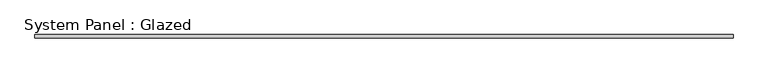
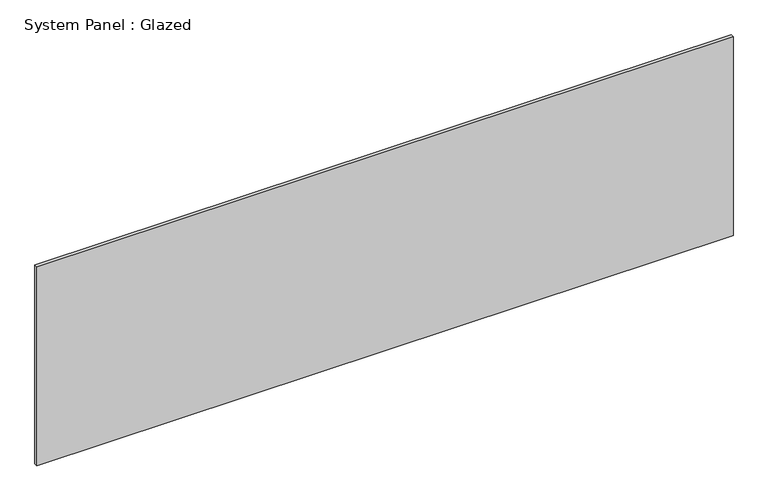
"""IFC4 building model written with IfcOpenShell, lengths in millimetres: plate geometry, System Panel : Glazed."""

from ifc_helpers import new_model, si_unit, origin, origin_with_axes, place, context, project, spatial, polyline, outline, extrude, source, transform, mapped, element, save


def system_panel_glazed_9244b5db(model_context):
    return source(origin(), model_context, "Body", "SweptSolid", [
        extrude(outline(polyline([(2522.7302398, 19.05), (-2522.7302398, 19.05), (-2522.7302398, 44.45), (2522.7302398, 44.45), (2522.7302398, 19.05)])), origin_with_axes(), (0.0, 0.0, 1.0), 1524.0),
    ])


if __name__ == "__main__":
    model = new_model("IFC4")
    model_context = context("Model", 3, world=origin())
    ifc_project = project(units=[si_unit("LENGTHUNIT", "METRE", prefix="MILLI")], contexts=[model_context])
    site = spatial("IfcSite", under=ifc_project)
    building = spatial("IfcBuilding", under=site)
    placement = place(None, origin())
    system_panel_glazed_shape = system_panel_glazed_9244b5db(model_context)
    element("IfcPlate", 1, ObjectType="System Panel : Glazed", at=placement, inside=building, context=model_context, shape_type="MappedRepresentation", body=[
        mapped(system_panel_glazed_shape, transform((0.0, 0.0, 0.0), x_axis=(1.0, 0.0, 0.0), y_axis=(0.0, 1.0, 0.0), z_axis=(0.0, 0.0, 1.0))),
    ])
    save(model, "model.ifc")

# Revit data of these elements
# Type "System Panel : Glazed"
#   Construction Type Id = "GSP4R"
#   Analytic Construction = "1/8 in Pilkington single glazing"
#   Visual Light Transmittance = 0.9
#   Solar Heat Gain Coefficient = 0.86
#   Heat Transfer Coefficient (U) = 1.18115 BTU/(h·ft²·°F)
# Element 1 (IfcPlate, "System Panel : Glazed")
#   Materials on its faces: "Glass"
# Materials
#   "Glass": class "Glass", colour RGB 0 128 192, transparency 0.75, Description = "Soda Lime Glass", Cost = 0
